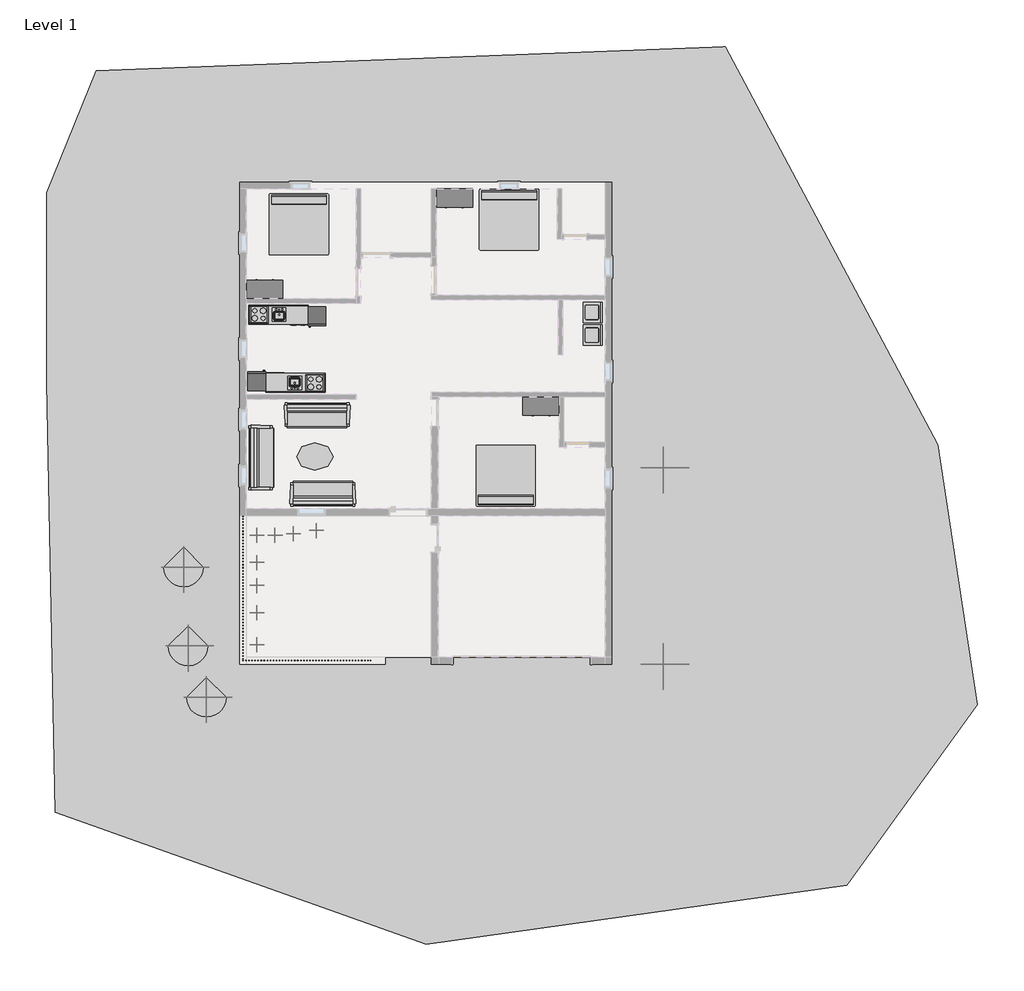
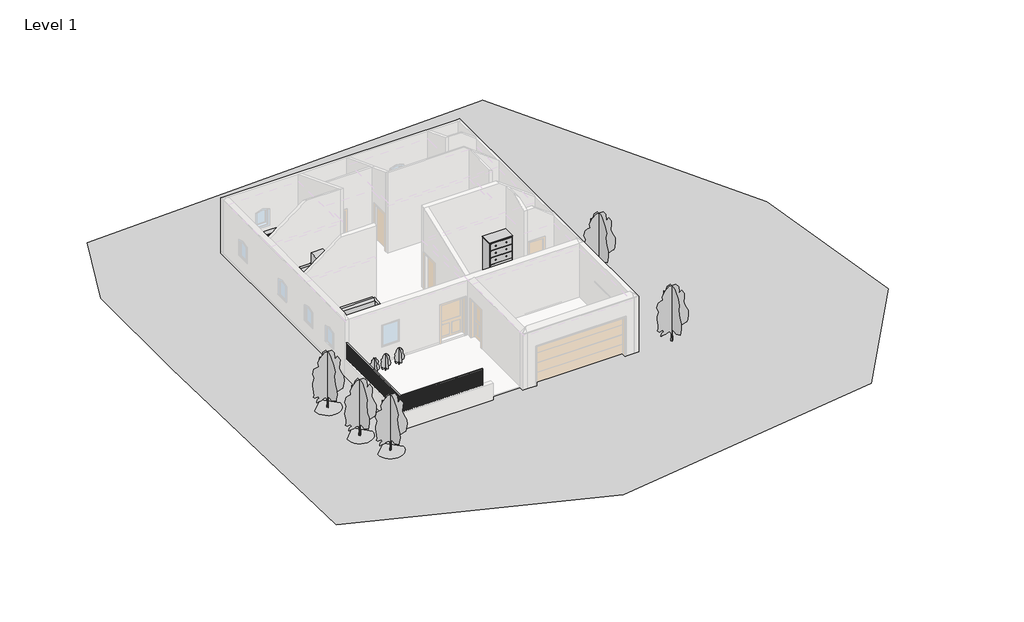
# One storey, part 3 of 3: 13 geographic elements, 12 furniture elements, 11 proxies, 2 flow terminals, 1 railing.
"""IFC4 building model written with IfcOpenShell, lengths in millimetres."""

from ifc_helpers import new_model, si_unit, frame, origin, place, context, project, spatial, polyline, outline, extrude, faceted_brep, triangles, transform, mapped, element, save
from components import proxy_a6faaae8, proxy_45b28599, kitchenette_medium_kitchenette_medium_844211aa, proxy_c523a7b7, proxy_718fa39f, flow_terminal_871c2e40, furniture_1fc5af50, furniture_c6510c7c, furniture_9fa109b2, furniture_aff9b2fb, furniture_b1c544a7, rpc_tree_deciduous_10_2_5dd3353f, rpc_tree_deciduous_red_ash_25_29d6c0be

model = new_model("IFC4")

# Units and contexts
model_context = context("Model", 3, world=origin())
ifc_project = project(units=[si_unit("LENGTHUNIT", "METRE", prefix="MILLI")], contexts=[model_context])

# Site, building, storey
site = spatial("IfcSite", under=ifc_project)
building = spatial("IfcBuilding", under=site)
storey = spatial("IfcBuildingStorey", under=building, Name="Level 1", Elevation=0.0)

# Proxies
placement = place(None, origin())
element("IfcBuildingElementProxy", 1, Name="Building Element Proxy", at=placement, inside=storey, context=model_context, shape_type="Tessellation", body=[
    triangles([(-17802.37034, 12771.1681366, 0.0), (3187.6458366, 13578.4769989, 0.0), (10269.9417389, 294.5849622, 0.0), (11590.9913361, -8365.631813, 0.0), (7224.187532, -14383.7487762, 0.0), (-6793.6207901, -16365.323172, 0.0), (-19160.1165344, -11961.8233521, 0.0), (-19453.6834991, 2386.2475147, 0.0), (-19453.6834991, 8697.9307159, 0.0)], [[2, 9, 8], [2, 1, 9], [8, 7, 6], [6, 5, 3], [3, 2, 8], [3, 5, 4], [3, 8, 6]], closed=False),
])
proxy_shape = proxy_a6faaae8(model_context)
element("IfcBuildingElementProxy", 2, Name="Cook Top-4 Unit2 : 22\" x 20\"", ObjectType="Cook Top-4 Unit2 : 22\" x 20\"", at=placement, inside=storey, context=model_context, shape_type="MappedRepresentation", body=[
    mapped(proxy_shape, transform((-12370.7368615, 4641.3670221, 152.4), x_axis=(1.0, 0.0, 0.0), y_axis=(0.0, 1.0, 0.0), z_axis=(0.0, 0.0, 1.0))),
])
element("IfcBuildingElementProxy", 3, Name="Cook Top-4 Unit2 : 22\" x 20\"", ObjectType="Cook Top-4 Unit2 : 22\" x 20\"", at=placement, inside=storey, context=model_context, shape_type="MappedRepresentation", body=[
    mapped(proxy_shape, transform((-10503.8368615, 2355.3670221, 152.4), x_axis=(-1.0, 0.0, 0.0), y_axis=(0.0, -1.0, 0.0), z_axis=(0.0, 0.0, 1.0))),
])
proxy_2_shape = proxy_45b28599(model_context)
element("IfcBuildingElementProxy", 4, Name="Dishwasher : 24\" x 24\" x 34\"", ObjectType="Dishwasher : 24\" x 24\" x 34\"", at=placement, inside=storey, context=model_context, shape_type="MappedRepresentation", body=[
    mapped(proxy_2_shape, transform((-11419.55433, 4349.5174573, 152.4), x_axis=(1.0, 0.0, 0.0), y_axis=(0.0, 1.0, 0.0), z_axis=(0.0, 0.0, 1.0))),
])
element("IfcBuildingElementProxy", 5, Name="Dishwasher : 24\" x 24\" x 34\"", ObjectType="Dishwasher : 24\" x 24\" x 34\"", at=placement, inside=storey, context=model_context, shape_type="MappedRepresentation", body=[
    mapped(proxy_2_shape, transform((-11455.019393, 2647.2165869, 152.4), x_axis=(-1.0, 0.0, 0.0), y_axis=(0.0, -1.0, 0.0), z_axis=(0.0, 0.0, 1.0))),
])
kitchenette_medium_kitchenette_medium_shape = kitchenette_medium_kitchenette_medium_844211aa(model_context)
element("IfcBuildingElementProxy", 6, Name="Kitchenette - Medium : Kitchenette - Medium", ObjectType="Kitchenette - Medium : Kitchenette - Medium", at=placement, inside=storey, context=model_context, shape_type="MappedRepresentation", body=[
    mapped(kitchenette_medium_kitchenette_medium_shape, transform((-12046.5745664, 4946.1670221, 152.4), x_axis=(1.0, 0.0, 0.0), y_axis=(0.0, 1.0, 0.0), z_axis=(0.0, 0.0, 1.0))),
])
element("IfcBuildingElementProxy", 7, Name="Kitchenette - Medium : Kitchenette - Medium", ObjectType="Kitchenette - Medium : Kitchenette - Medium", at=placement, inside=storey, context=model_context, shape_type="MappedRepresentation", body=[
    mapped(kitchenette_medium_kitchenette_medium_shape, transform((-10827.9991566, 2050.5670221, 152.4), x_axis=(-1.0, 0.0, 0.0), y_axis=(0.0, -1.0, 0.0), z_axis=(0.0, 0.0, 1.0))),
])
proxy_3_shape = proxy_c523a7b7(model_context)
element("IfcBuildingElementProxy", 8, Name="Refrigerator : 24\" x 25\" LH", ObjectType="Refrigerator : 24\" x 25\" LH", at=placement, inside=storey, context=model_context, shape_type="MappedRepresentation", body=[
    mapped(proxy_3_shape, transform((-10433.9868615, 4595.7180506, 152.4), x_axis=(1.0, 0.0, 0.0), y_axis=(0.0, 1.0, 0.0), z_axis=(0.0, 0.0, 1.0))),
])
element("IfcBuildingElementProxy", 9, Name="Refrigerator : 24\" x 25\" LH", ObjectType="Refrigerator : 24\" x 25\" LH", at=placement, inside=storey, context=model_context, shape_type="MappedRepresentation", body=[
    mapped(proxy_3_shape, transform((-12440.5868615, 2401.0159936, 152.4), x_axis=(-1.0, 0.0, 0.0), y_axis=(0.0, -1.0, 0.0), z_axis=(0.0, 0.0, 1.0))),
])
proxy_4_shape = proxy_718fa39f(model_context)
element("IfcBuildingElementProxy", 10, Name="Washer : 27\" x 25\" x 35\"", ObjectType="Washer : 27\" x 25\" x 35\"", at=placement, inside=storey, context=model_context, shape_type="MappedRepresentation", body=[
    mapped(proxy_4_shape, transform((-1511.9864263, 5136.6670221, 152.4), x_axis=(0.0, -1.0, 0.0), y_axis=(1.0, 0.0, 0.0), z_axis=(0.0, 0.0, 1.0))),
])
element("IfcBuildingElementProxy", 11, Name="Washer : 27\" x 25\" x 35\"", ObjectType="Washer : 27\" x 25\" x 35\"", at=placement, inside=storey, context=model_context, shape_type="MappedRepresentation", body=[
    mapped(proxy_4_shape, transform((-1511.9864263, 4373.3495536, 152.4), x_axis=(0.0, -1.0, 0.0), y_axis=(1.0, 0.0, 0.0), z_axis=(0.0, 0.0, 1.0))),
])

# Flow terminals
flow_terminal_shape = flow_terminal_871c2e40(model_context)
element("IfcFlowTerminal", 12, ObjectType="Sink Kitchen-Island : 18\" x 18\"", at=placement, inside=storey, context=model_context, shape_type="MappedRepresentation", body=[
    mapped(flow_terminal_shape, transform((-11713.3261021, 4639.021621, 138.0), x_axis=(1.0, 0.0, 0.0), y_axis=(0.0, 1.0, 0.0), z_axis=(0.0, 0.0, 1.0))),
])
element("IfcFlowTerminal", 13, ObjectType="Sink Kitchen-Island : 18\" x 18\"", at=placement, inside=storey, context=model_context, shape_type="MappedRepresentation", body=[
    mapped(flow_terminal_shape, transform((-11161.2476209, 2357.7124232, 138.0), x_axis=(-1.0, 0.0, 0.0), y_axis=(0.0, -1.0, 0.0), z_axis=(0.0, 0.0, 1.0))),
])

# Furniture
furniture_shape = furniture_1fc5af50(model_context)
element("IfcFurniture", 14, ObjectType="Bed-Standard : King 78\" x 80\"", at=placement, inside=storey, context=model_context, shape_type="MappedRepresentation", body=[
    mapped(furniture_shape, transform((-11308.7253861, 7696.8621041, 152.4), x_axis=(1.0, 0.0, 0.0), y_axis=(0.0, 1.0, 0.0), z_axis=(0.0, 0.0, 1.0))),
])
element("IfcFurniture", 15, ObjectType="Bed-Standard : King 78\" x 80\"", at=placement, inside=storey, context=model_context, shape_type="MappedRepresentation", body=[
    mapped(furniture_shape, transform((-4298.3253861, 7849.2621041, 152.4), x_axis=(1.0, 0.0, 0.0), y_axis=(0.0, 1.0, 0.0), z_axis=(0.0, 0.0, 1.0))),
])
element("IfcFurniture", 16, ObjectType="Bed-Standard : King 78\" x 80\"", at=placement, inside=storey, context=model_context, shape_type="MappedRepresentation", body=[
    mapped(furniture_shape, transform((-3869.6483369, -776.3280599, 152.4), x_axis=(-1.0000000000000002, 0.0, 0.0), y_axis=(0.0, -1.0000000000000002, 0.0), z_axis=(0.0, 0.0, 1.0))),
])
furniture_2_shape = furniture_c6510c7c(model_context)
element("IfcFurniture", 17, ObjectType="Counter Top w Sink Hole : 24\" Depth", at=placement, inside=storey, context=model_context, shape_type="MappedRepresentation", body=[
    mapped(furniture_2_shape, transform((-11513.1745664, 4946.1670221, 138.0), x_axis=(1.0, 0.0, 0.0), y_axis=(0.0, 1.0, 0.0), z_axis=(0.0, 0.0, 1.0))),
])
element("IfcFurniture", 18, ObjectType="Counter Top w Sink Hole : 24\" Depth", at=placement, inside=storey, context=model_context, shape_type="MappedRepresentation", body=[
    mapped(furniture_2_shape, transform((-11361.3991566, 2050.5670221, 138.0), x_axis=(-1.0, 0.0, 0.0), y_axis=(0.0, -1.0, 0.0), z_axis=(0.0, 0.0, 1.0))),
])
furniture_3_shape = furniture_9fa109b2(model_context)
element("IfcFurniture", 19, ObjectType="Dresser : 48\" x 72\" x 24\"", at=placement, inside=storey, context=model_context, shape_type="MappedRepresentation", body=[
    mapped(furniture_3_shape, transform((-12449.4301213, 5116.404068, 152.4), x_axis=(-1.0000000000000004, 0.0, 0.0), y_axis=(0.0, -1.0000000000000004, 0.0), z_axis=(0.0, 0.0, 1.0))),
])
element("IfcFurniture", 20, ObjectType="Dresser : 48\" x 72\" x 24\"", at=placement, inside=storey, context=model_context, shape_type="MappedRepresentation", body=[
    mapped(furniture_3_shape, transform((-5586.4436017, 8890.7299762, 152.4), x_axis=(1.0000000000000004, 0.0, 0.0), y_axis=(0.0, 1.0000000000000004, 0.0), z_axis=(0.0, 0.0, 1.0))),
])
element("IfcFurniture", 21, ObjectType="Dresser : 48\" x 72\" x 24\"", at=placement, inside=storey, context=model_context, shape_type="MappedRepresentation", body=[
    mapped(furniture_3_shape, transform((-2690.8436017, 1956.5299762, 152.4), x_axis=(1.0000000000000004, 0.0, 0.0), y_axis=(0.0, 1.0000000000000004, 0.0), z_axis=(0.0, 0.0, 1.0))),
])
furniture_4_shape = furniture_aff9b2fb(model_context)
element("IfcFurniture", 22, ObjectType="Sofa-Pensi : 84\"", at=placement, inside=storey, context=model_context, shape_type="MappedRepresentation", body=[
    mapped(furniture_4_shape, transform((-12017.4270254, -412.4392279, 152.4), x_axis=(0.0, 1.0000000000000002, 0.0), y_axis=(-1.0000000000000002, 0.0, 0.0), z_axis=(0.0, 0.0, 1.0))),
])
element("IfcFurniture", 23, ObjectType="Sofa-Pensi : 84\"", at=placement, inside=storey, context=model_context, shape_type="MappedRepresentation", body=[
    mapped(furniture_4_shape, transform((-10706.2431115, 1011.457186, 152.4), x_axis=(1.0000000000000007, 0.0, 0.0), y_axis=(0.0, 1.0000000000000007, 0.0), z_axis=(0.0, 0.0, 1.0))),
])
element("IfcFurniture", 24, ObjectType="Sofa-Pensi : 84\"", at=placement, inside=storey, context=model_context, shape_type="MappedRepresentation", body=[
    mapped(furniture_4_shape, transform((-9958.5306115, -1063.2231418, 152.4), x_axis=(-1.0000000000000004, 0.0, 0.0), y_axis=(0.0, -1.0000000000000004, 0.0), z_axis=(0.0, 0.0, 1.0))),
])
furniture_5_shape = furniture_b1c544a7(model_context)
element("IfcFurniture", 25, ObjectType="Table-Ellipse : 60\" x 48\"", at=placement, inside=storey, context=model_context, shape_type="MappedRepresentation", body=[
    mapped(furniture_5_shape, transform((-10503.8368615, -95.7329779, 152.4), x_axis=(0.0, -1.0000000000000004, 0.0), y_axis=(1.0000000000000004, 0.0, 0.0), z_axis=(0.0, 0.0, 1.0))),
])

# Geographic elements
rpc_tree_deciduous_10_2_shape = rpc_tree_deciduous_10_2_5dd3353f(model_context)
element("IfcGeographicElement", 26, ObjectType="RPC Tree - Deciduous : 10' 2", at=placement, inside=storey, context=model_context, shape_type="MappedRepresentation", body=[
    mapped(rpc_tree_deciduous_10_2_shape, transform((-14885.3368615, -3778.7329779, 0.0), x_axis=(1.0, 0.0, 0.0), y_axis=(0.0, 1.0, 0.0), z_axis=(0.0, 0.0, 1.0))),
])
element("IfcGeographicElement", 27, ObjectType="RPC Tree - Deciduous : 10' 2", at=placement, inside=storey, context=model_context, shape_type="MappedRepresentation", body=[
    mapped(rpc_tree_deciduous_10_2_shape, transform((-14732.9368615, -6407.6329779, 0.0), x_axis=(1.0, 0.0, 0.0), y_axis=(0.0, 1.0, 0.0), z_axis=(0.0, 0.0, 1.0))),
])
element("IfcGeographicElement", 28, ObjectType="RPC Tree - Deciduous : 10' 2", at=placement, inside=storey, context=model_context, shape_type="MappedRepresentation", body=[
    mapped(rpc_tree_deciduous_10_2_shape, transform((1116.6631385, -7017.2329779, 0.0), x_axis=(1.0, 0.0, 0.0), y_axis=(0.0, 1.0, 0.0), z_axis=(0.0, 0.0, 1.0))),
])
element("IfcGeographicElement", 29, ObjectType="RPC Tree - Deciduous : 10' 2", at=placement, inside=storey, context=model_context, shape_type="MappedRepresentation", body=[
    mapped(rpc_tree_deciduous_10_2_shape, transform((1116.6631385, -464.0329779, 0.0), x_axis=(1.0, 0.0, 0.0), y_axis=(0.0, 1.0, 0.0), z_axis=(0.0, 0.0, 1.0))),
])
element("IfcGeographicElement", 30, ObjectType="RPC Tree - Deciduous : 10' 2", at=placement, inside=storey, context=model_context, shape_type="MappedRepresentation", body=[
    mapped(rpc_tree_deciduous_10_2_shape, transform((-14123.3368615, -8122.1329779, 0.0), x_axis=(1.0, 0.0, 0.0), y_axis=(0.0, 1.0, 0.0), z_axis=(0.0, 0.0, 1.0))),
])
rpc_tree_deciduous_red_ash_25_shape = rpc_tree_deciduous_red_ash_25_29d6c0be(model_context)
element("IfcGeographicElement", 31, ObjectType="RPC Tree - Deciduous : Red Ash - 25'", at=placement, inside=storey, context=model_context, shape_type="MappedRepresentation", body=[
    mapped(rpc_tree_deciduous_red_ash_25_shape, transform((-12446.9368615, -2711.9329779, 50.8), x_axis=(1.0, 0.0, 0.0), y_axis=(0.0, 1.0, 0.0), z_axis=(0.0, 0.0, 1.0))),
])
element("IfcGeographicElement", 32, ObjectType="RPC Tree - Deciduous : Red Ash - 25'", at=placement, inside=storey, context=model_context, shape_type="MappedRepresentation", body=[
    mapped(rpc_tree_deciduous_red_ash_25_shape, transform((-12446.9368615, -3626.3329779, 50.8), x_axis=(1.0, 0.0, 0.0), y_axis=(0.0, 1.0, 0.0), z_axis=(0.0, 0.0, 1.0))),
])
element("IfcGeographicElement", 33, ObjectType="RPC Tree - Deciduous : Red Ash - 25'", at=placement, inside=storey, context=model_context, shape_type="MappedRepresentation", body=[
    mapped(rpc_tree_deciduous_red_ash_25_shape, transform((-12446.9368615, -4388.3329779, 50.8), x_axis=(1.0, 0.0, 0.0), y_axis=(0.0, 1.0, 0.0), z_axis=(0.0, 0.0, 1.0))),
])
element("IfcGeographicElement", 34, ObjectType="RPC Tree - Deciduous : Red Ash - 25'", at=placement, inside=storey, context=model_context, shape_type="MappedRepresentation", body=[
    mapped(rpc_tree_deciduous_red_ash_25_shape, transform((-12446.9368615, -5302.7329779, 50.8), x_axis=(1.0, 0.0, 0.0), y_axis=(0.0, 1.0, 0.0), z_axis=(0.0, 0.0, 1.0))),
])
element("IfcGeographicElement", 35, ObjectType="RPC Tree - Deciduous : Red Ash - 25'", at=placement, inside=storey, context=model_context, shape_type="MappedRepresentation", body=[
    mapped(rpc_tree_deciduous_red_ash_25_shape, transform((-12446.9368615, -6369.5329779, 50.8), x_axis=(1.0, 0.0, 0.0), y_axis=(0.0, 1.0, 0.0), z_axis=(0.0, 0.0, 1.0))),
])
element("IfcGeographicElement", 36, ObjectType="RPC Tree - Deciduous : Red Ash - 25'", at=placement, inside=storey, context=model_context, shape_type="MappedRepresentation", body=[
    mapped(rpc_tree_deciduous_red_ash_25_shape, transform((-11837.3368615, -2711.9329779, 50.8), x_axis=(1.0, 0.0, 0.0), y_axis=(0.0, 1.0, 0.0), z_axis=(0.0, 0.0, 1.0))),
])
element("IfcGeographicElement", 37, ObjectType="RPC Tree - Deciduous : Red Ash - 25'", at=placement, inside=storey, context=model_context, shape_type="MappedRepresentation", body=[
    mapped(rpc_tree_deciduous_red_ash_25_shape, transform((-11227.7368615, -2661.1329779, 50.8), x_axis=(1.0, 0.0, 0.0), y_axis=(0.0, 1.0, 0.0), z_axis=(0.0, 0.0, 1.0))),
])
element("IfcGeographicElement", 38, ObjectType="RPC Tree - Deciduous : Red Ash - 25'", at=placement, inside=storey, context=model_context, shape_type="MappedRepresentation", body=[
    mapped(rpc_tree_deciduous_red_ash_25_shape, transform((-10465.7368615, -2559.5329779, 50.8), x_axis=(1.0, 0.0, 0.0), y_axis=(0.0, 1.0, 0.0), z_axis=(0.0, 0.0, 1.0))),
])

# Railing
element("IfcRailing", 39, ObjectType="Handrail - Rectangular", at=placement, inside=storey, context=model_context, shape_type="SolidModel", body=[
    faceted_brep([(-12878.7368615, -2076.9329779, 1828.8), (-12878.7368615, -2076.9329779, 1778.0), (-12929.5368615, -2076.9329779, 1778.0), (-12929.5368615, -2076.9329779, 1828.8), (-12878.7368615, -6877.5329779, 1828.8), (-12878.7368615, -6877.5329779, 1778.0), (-12929.5368615, -6928.3329779, 1778.0), (-12929.5368615, -6928.3329779, 1828.8), (-8636.9368615, -6877.5329779, 1828.8), (-8636.9368615, -6928.3329779, 1828.8), (-8636.9368615, -6928.3329779, 1778.0), (-8636.9368615, -6877.5329779, 1778.0)], [[[0, 1, 2, 3]], [[1, 0, 4, 5]], [[2, 1, 5, 6]], [[3, 2, 6, 7]], [[0, 3, 7, 4]], [[8, 9, 10, 11]], [[5, 4, 8, 11]], [[6, 5, 11, 10]], [[7, 6, 10, 9]], [[4, 7, 9, 8]]]),
    extrude(outline(polyline([(-8748.0618615, -6912.4579779), (-8748.0618615, -6893.4079779), (-8729.0118615, -6893.4079779), (-8729.0118615, -6912.4579779), (-8748.0618615, -6912.4579779)])), frame((0.0, 0.0, 914.4), z_axis=(0.0, 0.0, 1.0), x_axis=(1.0, 0.0, 0.0)), (0.0, 0.0, 1.0), 863.6),
    extrude(outline(polyline([(-8849.6618615, -6912.4579779), (-8849.6618615, -6893.4079779), (-8830.6118615, -6893.4079779), (-8830.6118615, -6912.4579779), (-8849.6618615, -6912.4579779)])), frame((0.0, 0.0, 914.4), z_axis=(0.0, 0.0, 1.0), x_axis=(1.0, 0.0, 0.0)), (0.0, 0.0, 1.0), 863.6),
    extrude(outline(polyline([(-8951.2618615, -6912.4579779), (-8951.2618615, -6893.4079779), (-8932.2118615, -6893.4079779), (-8932.2118615, -6912.4579779), (-8951.2618615, -6912.4579779)])), frame((0.0, 0.0, 914.4), z_axis=(0.0, 0.0, 1.0), x_axis=(1.0, 0.0, 0.0)), (0.0, 0.0, 1.0), 863.6),
    extrude(outline(polyline([(-9052.8618615, -6912.4579779), (-9052.8618615, -6893.4079779), (-9033.8118615, -6893.4079779), (-9033.8118615, -6912.4579779), (-9052.8618615, -6912.4579779)])), frame((0.0, 0.0, 914.4), z_axis=(0.0, 0.0, 1.0), x_axis=(1.0, 0.0, 0.0)), (0.0, 0.0, 1.0), 863.6),
    extrude(outline(polyline([(-9154.4618615, -6912.4579779), (-9154.4618615, -6893.4079779), (-9135.4118615, -6893.4079779), (-9135.4118615, -6912.4579779), (-9154.4618615, -6912.4579779)])), frame((0.0, 0.0, 914.4), z_axis=(0.0, 0.0, 1.0), x_axis=(1.0, 0.0, 0.0)), (0.0, 0.0, 1.0), 863.6),
    extrude(outline(polyline([(-9256.0618615, -6912.4579779), (-9256.0618615, -6893.4079779), (-9237.0118615, -6893.4079779), (-9237.0118615, -6912.4579779), (-9256.0618615, -6912.4579779)])), frame((0.0, 0.0, 914.4), z_axis=(0.0, 0.0, 1.0), x_axis=(1.0, 0.0, 0.0)), (0.0, 0.0, 1.0), 863.6),
    extrude(outline(polyline([(-9357.6618615, -6912.4579779), (-9357.6618615, -6893.4079779), (-9338.6118615, -6893.4079779), (-9338.6118615, -6912.4579779), (-9357.6618615, -6912.4579779)])), frame((0.0, 0.0, 914.4), z_axis=(0.0, 0.0, 1.0), x_axis=(1.0, 0.0, 0.0)), (0.0, 0.0, 1.0), 863.6),
    extrude(outline(polyline([(-9459.2618615, -6912.4579779), (-9459.2618615, -6893.4079779), (-9440.2118615, -6893.4079779), (-9440.2118615, -6912.4579779), (-9459.2618615, -6912.4579779)])), frame((0.0, 0.0, 914.4), z_axis=(0.0, 0.0, 1.0), x_axis=(1.0, 0.0, 0.0)), (0.0, 0.0, 1.0), 863.6),
    extrude(outline(polyline([(-9560.8618615, -6912.4579779), (-9560.8618615, -6893.4079779), (-9541.8118615, -6893.4079779), (-9541.8118615, -6912.4579779), (-9560.8618615, -6912.4579779)])), frame((0.0, 0.0, 914.4), z_axis=(0.0, 0.0, 1.0), x_axis=(1.0, 0.0, 0.0)), (0.0, 0.0, 1.0), 863.6),
    extrude(outline(polyline([(-9662.4618615, -6912.4579779), (-9662.4618615, -6893.4079779), (-9643.4118615, -6893.4079779), (-9643.4118615, -6912.4579779), (-9662.4618615, -6912.4579779)])), frame((0.0, 0.0, 914.4), z_axis=(0.0, 0.0, 1.0), x_axis=(1.0, 0.0, 0.0)), (0.0, 0.0, 1.0), 863.6),
    extrude(outline(polyline([(-9764.0618615, -6912.4579779), (-9764.0618615, -6893.4079779), (-9745.0118615, -6893.4079779), (-9745.0118615, -6912.4579779), (-9764.0618615, -6912.4579779)])), frame((0.0, 0.0, 914.4), z_axis=(0.0, 0.0, 1.0), x_axis=(1.0, 0.0, 0.0)), (0.0, 0.0, 1.0), 863.6),
    extrude(outline(polyline([(-9865.6618615, -6912.4579779), (-9865.6618615, -6893.4079779), (-9846.6118615, -6893.4079779), (-9846.6118615, -6912.4579779), (-9865.6618615, -6912.4579779)])), frame((0.0, 0.0, 914.4), z_axis=(0.0, 0.0, 1.0), x_axis=(1.0, 0.0, 0.0)), (0.0, 0.0, 1.0), 863.6),
    extrude(outline(polyline([(-9967.2618615, -6912.4579779), (-9967.2618615, -6893.4079779), (-9948.2118615, -6893.4079779), (-9948.2118615, -6912.4579779), (-9967.2618615, -6912.4579779)])), frame((0.0, 0.0, 914.4), z_axis=(0.0, 0.0, 1.0), x_axis=(1.0, 0.0, 0.0)), (0.0, 0.0, 1.0), 863.6),
    extrude(outline(polyline([(-10068.8618615, -6912.4579779), (-10068.8618615, -6893.4079779), (-10049.8118615, -6893.4079779), (-10049.8118615, -6912.4579779), (-10068.8618615, -6912.4579779)])), frame((0.0, 0.0, 914.4), z_axis=(0.0, 0.0, 1.0), x_axis=(1.0, 0.0, 0.0)), (0.0, 0.0, 1.0), 863.6),
    extrude(outline(polyline([(-10170.4618615, -6912.4579779), (-10170.4618615, -6893.4079779), (-10151.4118615, -6893.4079779), (-10151.4118615, -6912.4579779), (-10170.4618615, -6912.4579779)])), frame((0.0, 0.0, 914.4), z_axis=(0.0, 0.0, 1.0), x_axis=(1.0, 0.0, 0.0)), (0.0, 0.0, 1.0), 863.6),
    extrude(outline(polyline([(-10272.0618615, -6912.4579779), (-10272.0618615, -6893.4079779), (-10253.0118615, -6893.4079779), (-10253.0118615, -6912.4579779), (-10272.0618615, -6912.4579779)])), frame((0.0, 0.0, 914.4), z_axis=(0.0, 0.0, 1.0), x_axis=(1.0, 0.0, 0.0)), (0.0, 0.0, 1.0), 863.6),
    extrude(outline(polyline([(-10373.6618615, -6912.4579779), (-10373.6618615, -6893.4079779), (-10354.6118615, -6893.4079779), (-10354.6118615, -6912.4579779), (-10373.6618615, -6912.4579779)])), frame((0.0, 0.0, 914.4), z_axis=(0.0, 0.0, 1.0), x_axis=(1.0, 0.0, 0.0)), (0.0, 0.0, 1.0), 863.6),
    extrude(outline(polyline([(-10475.2618615, -6912.4579779), (-10475.2618615, -6893.4079779), (-10456.2118615, -6893.4079779), (-10456.2118615, -6912.4579779), (-10475.2618615, -6912.4579779)])), frame((0.0, 0.0, 914.4), z_axis=(0.0, 0.0, 1.0), x_axis=(1.0, 0.0, 0.0)), (0.0, 0.0, 1.0), 863.6),
    extrude(outline(polyline([(-10576.8618615, -6912.4579779), (-10576.8618615, -6893.4079779), (-10557.8118615, -6893.4079779), (-10557.8118615, -6912.4579779), (-10576.8618615, -6912.4579779)])), frame((0.0, 0.0, 914.4), z_axis=(0.0, 0.0, 1.0), x_axis=(1.0, 0.0, 0.0)), (0.0, 0.0, 1.0), 863.6),
    extrude(outline(polyline([(-10678.4618615, -6912.4579779), (-10678.4618615, -6893.4079779), (-10659.4118615, -6893.4079779), (-10659.4118615, -6912.4579779), (-10678.4618615, -6912.4579779)])), frame((0.0, 0.0, 914.4), z_axis=(0.0, 0.0, 1.0), x_axis=(1.0, 0.0, 0.0)), (0.0, 0.0, 1.0), 863.6),
    extrude(outline(polyline([(-10780.0618615, -6912.4579779), (-10780.0618615, -6893.4079779), (-10761.0118615, -6893.4079779), (-10761.0118615, -6912.4579779), (-10780.0618615, -6912.4579779)])), frame((0.0, 0.0, 914.4), z_axis=(0.0, 0.0, 1.0), x_axis=(1.0, 0.0, 0.0)), (0.0, 0.0, 1.0), 863.6),
    extrude(outline(polyline([(-10881.6618615, -6912.4579779), (-10881.6618615, -6893.4079779), (-10862.6118615, -6893.4079779), (-10862.6118615, -6912.4579779), (-10881.6618615, -6912.4579779)])), frame((0.0, 0.0, 914.4), z_axis=(0.0, 0.0, 1.0), x_axis=(1.0, 0.0, 0.0)), (0.0, 0.0, 1.0), 863.6),
    extrude(outline(polyline([(-10983.2618615, -6912.4579779), (-10983.2618615, -6893.4079779), (-10964.2118615, -6893.4079779), (-10964.2118615, -6912.4579779), (-10983.2618615, -6912.4579779)])), frame((0.0, 0.0, 914.4), z_axis=(0.0, 0.0, 1.0), x_axis=(1.0, 0.0, 0.0)), (0.0, 0.0, 1.0), 863.6),
    extrude(outline(polyline([(-11084.8618615, -6912.4579779), (-11084.8618615, -6893.4079779), (-11065.8118615, -6893.4079779), (-11065.8118615, -6912.4579779), (-11084.8618615, -6912.4579779)])), frame((0.0, 0.0, 914.4), z_axis=(0.0, 0.0, 1.0), x_axis=(1.0, 0.0, 0.0)), (0.0, 0.0, 1.0), 863.6),
    extrude(outline(polyline([(-11186.4618615, -6912.4579779), (-11186.4618615, -6893.4079779), (-11167.4118615, -6893.4079779), (-11167.4118615, -6912.4579779), (-11186.4618615, -6912.4579779)])), frame((0.0, 0.0, 914.4), z_axis=(0.0, 0.0, 1.0), x_axis=(1.0, 0.0, 0.0)), (0.0, 0.0, 1.0), 863.6),
    extrude(outline(polyline([(-11288.0618615, -6912.4579779), (-11288.0618615, -6893.4079779), (-11269.0118615, -6893.4079779), (-11269.0118615, -6912.4579779), (-11288.0618615, -6912.4579779)])), frame((0.0, 0.0, 914.4), z_axis=(0.0, 0.0, 1.0), x_axis=(1.0, 0.0, 0.0)), (0.0, 0.0, 1.0), 863.6),
    extrude(outline(polyline([(-11389.6618615, -6912.4579779), (-11389.6618615, -6893.4079779), (-11370.6118615, -6893.4079779), (-11370.6118615, -6912.4579779), (-11389.6618615, -6912.4579779)])), frame((0.0, 0.0, 914.4), z_axis=(0.0, 0.0, 1.0), x_axis=(1.0, 0.0, 0.0)), (0.0, 0.0, 1.0), 863.6),
    extrude(outline(polyline([(-11491.2618615, -6912.4579779), (-11491.2618615, -6893.4079779), (-11472.2118615, -6893.4079779), (-11472.2118615, -6912.4579779), (-11491.2618615, -6912.4579779)])), frame((0.0, 0.0, 914.4), z_axis=(0.0, 0.0, 1.0), x_axis=(1.0, 0.0, 0.0)), (0.0, 0.0, 1.0), 863.6),
    extrude(outline(polyline([(-11592.8618615, -6912.4579779), (-11592.8618615, -6893.4079779), (-11573.8118615, -6893.4079779), (-11573.8118615, -6912.4579779), (-11592.8618615, -6912.4579779)])), frame((0.0, 0.0, 914.4), z_axis=(0.0, 0.0, 1.0), x_axis=(1.0, 0.0, 0.0)), (0.0, 0.0, 1.0), 863.6),
    extrude(outline(polyline([(-11694.4618615, -6912.4579779), (-11694.4618615, -6893.4079779), (-11675.4118615, -6893.4079779), (-11675.4118615, -6912.4579779), (-11694.4618615, -6912.4579779)])), frame((0.0, 0.0, 914.4), z_axis=(0.0, 0.0, 1.0), x_axis=(1.0, 0.0, 0.0)), (0.0, 0.0, 1.0), 863.6),
    extrude(outline(polyline([(-11796.0618615, -6912.4579779), (-11796.0618615, -6893.4079779), (-11777.0118615, -6893.4079779), (-11777.0118615, -6912.4579779), (-11796.0618615, -6912.4579779)])), frame((0.0, 0.0, 914.4), z_axis=(0.0, 0.0, 1.0), x_axis=(1.0, 0.0, 0.0)), (0.0, 0.0, 1.0), 863.6),
    extrude(outline(polyline([(-11897.6618615, -6912.4579779), (-11897.6618615, -6893.4079779), (-11878.6118615, -6893.4079779), (-11878.6118615, -6912.4579779), (-11897.6618615, -6912.4579779)])), frame((0.0, 0.0, 914.4), z_axis=(0.0, 0.0, 1.0), x_axis=(1.0, 0.0, 0.0)), (0.0, 0.0, 1.0), 863.6),
    extrude(outline(polyline([(-11999.2618615, -6912.4579779), (-11999.2618615, -6893.4079779), (-11980.2118615, -6893.4079779), (-11980.2118615, -6912.4579779), (-11999.2618615, -6912.4579779)])), frame((0.0, 0.0, 914.4), z_axis=(0.0, 0.0, 1.0), x_axis=(1.0, 0.0, 0.0)), (0.0, 0.0, 1.0), 863.6),
    extrude(outline(polyline([(-12100.8618615, -6912.4579779), (-12100.8618615, -6893.4079779), (-12081.8118615, -6893.4079779), (-12081.8118615, -6912.4579779), (-12100.8618615, -6912.4579779)])), frame((0.0, 0.0, 914.4), z_axis=(0.0, 0.0, 1.0), x_axis=(1.0, 0.0, 0.0)), (0.0, 0.0, 1.0), 863.6),
    extrude(outline(polyline([(-12202.4618615, -6912.4579779), (-12202.4618615, -6893.4079779), (-12183.4118615, -6893.4079779), (-12183.4118615, -6912.4579779), (-12202.4618615, -6912.4579779)])), frame((0.0, 0.0, 914.4), z_axis=(0.0, 0.0, 1.0), x_axis=(1.0, 0.0, 0.0)), (0.0, 0.0, 1.0), 863.6),
    extrude(outline(polyline([(-12304.0618615, -6912.4579779), (-12304.0618615, -6893.4079779), (-12285.0118615, -6893.4079779), (-12285.0118615, -6912.4579779), (-12304.0618615, -6912.4579779)])), frame((0.0, 0.0, 914.4), z_axis=(0.0, 0.0, 1.0), x_axis=(1.0, 0.0, 0.0)), (0.0, 0.0, 1.0), 863.6),
    extrude(outline(polyline([(-12405.6618615, -6912.4579779), (-12405.6618615, -6893.4079779), (-12386.6118615, -6893.4079779), (-12386.6118615, -6912.4579779), (-12405.6618615, -6912.4579779)])), frame((0.0, 0.0, 914.4), z_axis=(0.0, 0.0, 1.0), x_axis=(1.0, 0.0, 0.0)), (0.0, 0.0, 1.0), 863.6),
    extrude(outline(polyline([(-12507.2618615, -6912.4579779), (-12507.2618615, -6893.4079779), (-12488.2118615, -6893.4079779), (-12488.2118615, -6912.4579779), (-12507.2618615, -6912.4579779)])), frame((0.0, 0.0, 914.4), z_axis=(0.0, 0.0, 1.0), x_axis=(1.0, 0.0, 0.0)), (0.0, 0.0, 1.0), 863.6),
    extrude(outline(polyline([(-12608.8618615, -6912.4579779), (-12608.8618615, -6893.4079779), (-12589.8118615, -6893.4079779), (-12589.8118615, -6912.4579779), (-12608.8618615, -6912.4579779)])), frame((0.0, 0.0, 914.4), z_axis=(0.0, 0.0, 1.0), x_axis=(1.0, 0.0, 0.0)), (0.0, 0.0, 1.0), 863.6),
    extrude(outline(polyline([(-12710.4618615, -6912.4579779), (-12710.4618615, -6893.4079779), (-12691.4118615, -6893.4079779), (-12691.4118615, -6912.4579779), (-12710.4618615, -6912.4579779)])), frame((0.0, 0.0, 914.4), z_axis=(0.0, 0.0, 1.0), x_axis=(1.0, 0.0, 0.0)), (0.0, 0.0, 1.0), 863.6),
    extrude(outline(polyline([(-12812.0618615, -6912.4579779), (-12812.0618615, -6893.4079779), (-12793.0118615, -6893.4079779), (-12793.0118615, -6912.4579779), (-12812.0618615, -6912.4579779)])), frame((0.0, 0.0, 914.4), z_axis=(0.0, 0.0, 1.0), x_axis=(1.0, 0.0, 0.0)), (0.0, 0.0, 1.0), 863.6),
    extrude(outline(polyline([(-12913.6618615, -6842.6079779), (-12894.6118615, -6842.6079779), (-12894.6118615, -6861.6579779), (-12913.6618615, -6861.6579779), (-12913.6618615, -6842.6079779)])), frame((0.0, 0.0, 914.4), z_axis=(0.0, 0.0, 1.0), x_axis=(1.0, 0.0, 0.0)), (0.0, 0.0, 1.0), 863.6),
    extrude(outline(polyline([(-12913.6618615, -6741.0079779), (-12894.6118615, -6741.0079779), (-12894.6118615, -6760.0579779), (-12913.6618615, -6760.0579779), (-12913.6618615, -6741.0079779)])), frame((0.0, 0.0, 914.4), z_axis=(0.0, 0.0, 1.0), x_axis=(1.0, 0.0, 0.0)), (0.0, 0.0, 1.0), 863.6),
    extrude(outline(polyline([(-12913.6618615, -6639.4079779), (-12894.6118615, -6639.4079779), (-12894.6118615, -6658.4579779), (-12913.6618615, -6658.4579779), (-12913.6618615, -6639.4079779)])), frame((0.0, 0.0, 914.4), z_axis=(0.0, 0.0, 1.0), x_axis=(1.0, 0.0, 0.0)), (0.0, 0.0, 1.0), 863.6),
    extrude(outline(polyline([(-12913.6618615, -6537.8079779), (-12894.6118615, -6537.8079779), (-12894.6118615, -6556.8579779), (-12913.6618615, -6556.8579779), (-12913.6618615, -6537.8079779)])), frame((0.0, 0.0, 914.4), z_axis=(0.0, 0.0, 1.0), x_axis=(1.0, 0.0, 0.0)), (0.0, 0.0, 1.0), 863.6),
    extrude(outline(polyline([(-12913.6618615, -6436.2079779), (-12894.6118615, -6436.2079779), (-12894.6118615, -6455.2579779), (-12913.6618615, -6455.2579779), (-12913.6618615, -6436.2079779)])), frame((0.0, 0.0, 914.4), z_axis=(0.0, 0.0, 1.0), x_axis=(1.0, 0.0, 0.0)), (0.0, 0.0, 1.0), 863.6),
    extrude(outline(polyline([(-12913.6618615, -6334.6079779), (-12894.6118615, -6334.6079779), (-12894.6118615, -6353.6579779), (-12913.6618615, -6353.6579779), (-12913.6618615, -6334.6079779)])), frame((0.0, 0.0, 914.4), z_axis=(0.0, 0.0, 1.0), x_axis=(1.0, 0.0, 0.0)), (0.0, 0.0, 1.0), 863.6),
    extrude(outline(polyline([(-12913.6618615, -6233.0079779), (-12894.6118615, -6233.0079779), (-12894.6118615, -6252.0579779), (-12913.6618615, -6252.0579779), (-12913.6618615, -6233.0079779)])), frame((0.0, 0.0, 914.4), z_axis=(0.0, 0.0, 1.0), x_axis=(1.0, 0.0, 0.0)), (0.0, 0.0, 1.0), 863.6),
    extrude(outline(polyline([(-12913.6618615, -6131.4079779), (-12894.6118615, -6131.4079779), (-12894.6118615, -6150.4579779), (-12913.6618615, -6150.4579779), (-12913.6618615, -6131.4079779)])), frame((0.0, 0.0, 914.4), z_axis=(0.0, 0.0, 1.0), x_axis=(1.0, 0.0, 0.0)), (0.0, 0.0, 1.0), 863.6),
    extrude(outline(polyline([(-12913.6618615, -6029.8079779), (-12894.6118615, -6029.8079779), (-12894.6118615, -6048.8579779), (-12913.6618615, -6048.8579779), (-12913.6618615, -6029.8079779)])), frame((0.0, 0.0, 914.4), z_axis=(0.0, 0.0, 1.0), x_axis=(1.0, 0.0, 0.0)), (0.0, 0.0, 1.0), 863.6),
    extrude(outline(polyline([(-12913.6618615, -5928.2079779), (-12894.6118615, -5928.2079779), (-12894.6118615, -5947.2579779), (-12913.6618615, -5947.2579779), (-12913.6618615, -5928.2079779)])), frame((0.0, 0.0, 914.4), z_axis=(0.0, 0.0, 1.0), x_axis=(1.0, 0.0, 0.0)), (0.0, 0.0, 1.0), 863.6),
    extrude(outline(polyline([(-12913.6618615, -5826.6079779), (-12894.6118615, -5826.6079779), (-12894.6118615, -5845.6579779), (-12913.6618615, -5845.6579779), (-12913.6618615, -5826.6079779)])), frame((0.0, 0.0, 914.4), z_axis=(0.0, 0.0, 1.0), x_axis=(1.0, 0.0, 0.0)), (0.0, 0.0, 1.0), 863.6),
    extrude(outline(polyline([(-12913.6618615, -5725.0079779), (-12894.6118615, -5725.0079779), (-12894.6118615, -5744.0579779), (-12913.6618615, -5744.0579779), (-12913.6618615, -5725.0079779)])), frame((0.0, 0.0, 914.4), z_axis=(0.0, 0.0, 1.0), x_axis=(1.0, 0.0, 0.0)), (0.0, 0.0, 1.0), 863.6),
    extrude(outline(polyline([(-12913.6618615, -5623.4079779), (-12894.6118615, -5623.4079779), (-12894.6118615, -5642.4579779), (-12913.6618615, -5642.4579779), (-12913.6618615, -5623.4079779)])), frame((0.0, 0.0, 914.4), z_axis=(0.0, 0.0, 1.0), x_axis=(1.0, 0.0, 0.0)), (0.0, 0.0, 1.0), 863.6),
    extrude(outline(polyline([(-12913.6618615, -5521.8079779), (-12894.6118615, -5521.8079779), (-12894.6118615, -5540.8579779), (-12913.6618615, -5540.8579779), (-12913.6618615, -5521.8079779)])), frame((0.0, 0.0, 914.4), z_axis=(0.0, 0.0, 1.0), x_axis=(1.0, 0.0, 0.0)), (0.0, 0.0, 1.0), 863.6),
    extrude(outline(polyline([(-12913.6618615, -5420.2079779), (-12894.6118615, -5420.2079779), (-12894.6118615, -5439.2579779), (-12913.6618615, -5439.2579779), (-12913.6618615, -5420.2079779)])), frame((0.0, 0.0, 914.4), z_axis=(0.0, 0.0, 1.0), x_axis=(1.0, 0.0, 0.0)), (0.0, 0.0, 1.0), 863.6),
    extrude(outline(polyline([(-12913.6618615, -5318.6079779), (-12894.6118615, -5318.6079779), (-12894.6118615, -5337.6579779), (-12913.6618615, -5337.6579779), (-12913.6618615, -5318.6079779)])), frame((0.0, 0.0, 914.4), z_axis=(0.0, 0.0, 1.0), x_axis=(1.0, 0.0, 0.0)), (0.0, 0.0, 1.0), 863.6),
    extrude(outline(polyline([(-12913.6618615, -5217.0079779), (-12894.6118615, -5217.0079779), (-12894.6118615, -5236.0579779), (-12913.6618615, -5236.0579779), (-12913.6618615, -5217.0079779)])), frame((0.0, 0.0, 914.4), z_axis=(0.0, 0.0, 1.0), x_axis=(1.0, 0.0, 0.0)), (0.0, 0.0, 1.0), 863.6),
    extrude(outline(polyline([(-12913.6618615, -5115.4079779), (-12894.6118615, -5115.4079779), (-12894.6118615, -5134.4579779), (-12913.6618615, -5134.4579779), (-12913.6618615, -5115.4079779)])), frame((0.0, 0.0, 914.4), z_axis=(0.0, 0.0, 1.0), x_axis=(1.0, 0.0, 0.0)), (0.0, 0.0, 1.0), 863.6),
    extrude(outline(polyline([(-12913.6618615, -5013.8079779), (-12894.6118615, -5013.8079779), (-12894.6118615, -5032.8579779), (-12913.6618615, -5032.8579779), (-12913.6618615, -5013.8079779)])), frame((0.0, 0.0, 914.4), z_axis=(0.0, 0.0, 1.0), x_axis=(1.0, 0.0, 0.0)), (0.0, 0.0, 1.0), 863.6),
    extrude(outline(polyline([(-12913.6618615, -4912.2079779), (-12894.6118615, -4912.2079779), (-12894.6118615, -4931.2579779), (-12913.6618615, -4931.2579779), (-12913.6618615, -4912.2079779)])), frame((0.0, 0.0, 914.4), z_axis=(0.0, 0.0, 1.0), x_axis=(1.0, 0.0, 0.0)), (0.0, 0.0, 1.0), 863.6),
    extrude(outline(polyline([(-12913.6618615, -4810.6079779), (-12894.6118615, -4810.6079779), (-12894.6118615, -4829.6579779), (-12913.6618615, -4829.6579779), (-12913.6618615, -4810.6079779)])), frame((0.0, 0.0, 914.4), z_axis=(0.0, 0.0, 1.0), x_axis=(1.0, 0.0, 0.0)), (0.0, 0.0, 1.0), 863.6),
    extrude(outline(polyline([(-12913.6618615, -4709.0079779), (-12894.6118615, -4709.0079779), (-12894.6118615, -4728.0579779), (-12913.6618615, -4728.0579779), (-12913.6618615, -4709.0079779)])), frame((0.0, 0.0, 914.4), z_axis=(0.0, 0.0, 1.0), x_axis=(1.0, 0.0, 0.0)), (0.0, 0.0, 1.0), 863.6),
    extrude(outline(polyline([(-12913.6618615, -4607.4079779), (-12894.6118615, -4607.4079779), (-12894.6118615, -4626.4579779), (-12913.6618615, -4626.4579779), (-12913.6618615, -4607.4079779)])), frame((0.0, 0.0, 914.4), z_axis=(0.0, 0.0, 1.0), x_axis=(1.0, 0.0, 0.0)), (0.0, 0.0, 1.0), 863.6),
    extrude(outline(polyline([(-12913.6618615, -4505.8079779), (-12894.6118615, -4505.8079779), (-12894.6118615, -4524.8579779), (-12913.6618615, -4524.8579779), (-12913.6618615, -4505.8079779)])), frame((0.0, 0.0, 914.4), z_axis=(0.0, 0.0, 1.0), x_axis=(1.0, 0.0, 0.0)), (0.0, 0.0, 1.0), 863.6),
    extrude(outline(polyline([(-12913.6618615, -4404.2079779), (-12894.6118615, -4404.2079779), (-12894.6118615, -4423.2579779), (-12913.6618615, -4423.2579779), (-12913.6618615, -4404.2079779)])), frame((0.0, 0.0, 914.4), z_axis=(0.0, 0.0, 1.0), x_axis=(1.0, 0.0, 0.0)), (0.0, 0.0, 1.0), 863.6),
    extrude(outline(polyline([(-12913.6618615, -4302.6079779), (-12894.6118615, -4302.6079779), (-12894.6118615, -4321.6579779), (-12913.6618615, -4321.6579779), (-12913.6618615, -4302.6079779)])), frame((0.0, 0.0, 914.4), z_axis=(0.0, 0.0, 1.0), x_axis=(1.0, 0.0, 0.0)), (0.0, 0.0, 1.0), 863.6),
    extrude(outline(polyline([(-12913.6618615, -4201.0079779), (-12894.6118615, -4201.0079779), (-12894.6118615, -4220.0579779), (-12913.6618615, -4220.0579779), (-12913.6618615, -4201.0079779)])), frame((0.0, 0.0, 914.4), z_axis=(0.0, 0.0, 1.0), x_axis=(1.0, 0.0, 0.0)), (0.0, 0.0, 1.0), 863.6),
    extrude(outline(polyline([(-12913.6618615, -4099.4079779), (-12894.6118615, -4099.4079779), (-12894.6118615, -4118.4579779), (-12913.6618615, -4118.4579779), (-12913.6618615, -4099.4079779)])), frame((0.0, 0.0, 914.4), z_axis=(0.0, 0.0, 1.0), x_axis=(1.0, 0.0, 0.0)), (0.0, 0.0, 1.0), 863.6),
    extrude(outline(polyline([(-12913.6618615, -3997.8079779), (-12894.6118615, -3997.8079779), (-12894.6118615, -4016.8579779), (-12913.6618615, -4016.8579779), (-12913.6618615, -3997.8079779)])), frame((0.0, 0.0, 914.4), z_axis=(0.0, 0.0, 1.0), x_axis=(1.0, 0.0, 0.0)), (0.0, 0.0, 1.0), 863.6),
    extrude(outline(polyline([(-12913.6618615, -3896.2079779), (-12894.6118615, -3896.2079779), (-12894.6118615, -3915.2579779), (-12913.6618615, -3915.2579779), (-12913.6618615, -3896.2079779)])), frame((0.0, 0.0, 914.4), z_axis=(0.0, 0.0, 1.0), x_axis=(1.0, 0.0, 0.0)), (0.0, 0.0, 1.0), 863.6),
    extrude(outline(polyline([(-12913.6618615, -3794.6079779), (-12894.6118615, -3794.6079779), (-12894.6118615, -3813.6579779), (-12913.6618615, -3813.6579779), (-12913.6618615, -3794.6079779)])), frame((0.0, 0.0, 914.4), z_axis=(0.0, 0.0, 1.0), x_axis=(1.0, 0.0, 0.0)), (0.0, 0.0, 1.0), 863.6),
    extrude(outline(polyline([(-12913.6618615, -3693.0079779), (-12894.6118615, -3693.0079779), (-12894.6118615, -3712.0579779), (-12913.6618615, -3712.0579779), (-12913.6618615, -3693.0079779)])), frame((0.0, 0.0, 914.4), z_axis=(0.0, 0.0, 1.0), x_axis=(1.0, 0.0, 0.0)), (0.0, 0.0, 1.0), 863.6),
    extrude(outline(polyline([(-12913.6618615, -3591.4079779), (-12894.6118615, -3591.4079779), (-12894.6118615, -3610.4579779), (-12913.6618615, -3610.4579779), (-12913.6618615, -3591.4079779)])), frame((0.0, 0.0, 914.4), z_axis=(0.0, 0.0, 1.0), x_axis=(1.0, 0.0, 0.0)), (0.0, 0.0, 1.0), 863.6),
    extrude(outline(polyline([(-12913.6618615, -3489.8079779), (-12894.6118615, -3489.8079779), (-12894.6118615, -3508.8579779), (-12913.6618615, -3508.8579779), (-12913.6618615, -3489.8079779)])), frame((0.0, 0.0, 914.4), z_axis=(0.0, 0.0, 1.0), x_axis=(1.0, 0.0, 0.0)), (0.0, 0.0, 1.0), 863.6),
    extrude(outline(polyline([(-12913.6618615, -3388.2079779), (-12894.6118615, -3388.2079779), (-12894.6118615, -3407.2579779), (-12913.6618615, -3407.2579779), (-12913.6618615, -3388.2079779)])), frame((0.0, 0.0, 914.4), z_axis=(0.0, 0.0, 1.0), x_axis=(1.0, 0.0, 0.0)), (0.0, 0.0, 1.0), 863.6),
    extrude(outline(polyline([(-12913.6618615, -3286.6079779), (-12894.6118615, -3286.6079779), (-12894.6118615, -3305.6579779), (-12913.6618615, -3305.6579779), (-12913.6618615, -3286.6079779)])), frame((0.0, 0.0, 914.4), z_axis=(0.0, 0.0, 1.0), x_axis=(1.0, 0.0, 0.0)), (0.0, 0.0, 1.0), 863.6),
    extrude(outline(polyline([(-12913.6618615, -3185.0079779), (-12894.6118615, -3185.0079779), (-12894.6118615, -3204.0579779), (-12913.6618615, -3204.0579779), (-12913.6618615, -3185.0079779)])), frame((0.0, 0.0, 914.4), z_axis=(0.0, 0.0, 1.0), x_axis=(1.0, 0.0, 0.0)), (0.0, 0.0, 1.0), 863.6),
    extrude(outline(polyline([(-12913.6618615, -3083.4079779), (-12894.6118615, -3083.4079779), (-12894.6118615, -3102.4579779), (-12913.6618615, -3102.4579779), (-12913.6618615, -3083.4079779)])), frame((0.0, 0.0, 914.4), z_axis=(0.0, 0.0, 1.0), x_axis=(1.0, 0.0, 0.0)), (0.0, 0.0, 1.0), 863.6),
    extrude(outline(polyline([(-12913.6618615, -2981.8079779), (-12894.6118615, -2981.8079779), (-12894.6118615, -3000.8579779), (-12913.6618615, -3000.8579779), (-12913.6618615, -2981.8079779)])), frame((0.0, 0.0, 914.4), z_axis=(0.0, 0.0, 1.0), x_axis=(1.0, 0.0, 0.0)), (0.0, 0.0, 1.0), 863.6),
    extrude(outline(polyline([(-12913.6618615, -2880.2079779), (-12894.6118615, -2880.2079779), (-12894.6118615, -2899.2579779), (-12913.6618615, -2899.2579779), (-12913.6618615, -2880.2079779)])), frame((0.0, 0.0, 914.4), z_axis=(0.0, 0.0, 1.0), x_axis=(1.0, 0.0, 0.0)), (0.0, 0.0, 1.0), 863.6),
    extrude(outline(polyline([(-12913.6618615, -2778.6079779), (-12894.6118615, -2778.6079779), (-12894.6118615, -2797.6579779), (-12913.6618615, -2797.6579779), (-12913.6618615, -2778.6079779)])), frame((0.0, 0.0, 914.4), z_axis=(0.0, 0.0, 1.0), x_axis=(1.0, 0.0, 0.0)), (0.0, 0.0, 1.0), 863.6),
    extrude(outline(polyline([(-12913.6618615, -2677.0079779), (-12894.6118615, -2677.0079779), (-12894.6118615, -2696.0579779), (-12913.6618615, -2696.0579779), (-12913.6618615, -2677.0079779)])), frame((0.0, 0.0, 914.4), z_axis=(0.0, 0.0, 1.0), x_axis=(1.0, 0.0, 0.0)), (0.0, 0.0, 1.0), 863.6),
    extrude(outline(polyline([(-12913.6618615, -2575.4079779), (-12894.6118615, -2575.4079779), (-12894.6118615, -2594.4579779), (-12913.6618615, -2594.4579779), (-12913.6618615, -2575.4079779)])), frame((0.0, 0.0, 914.4), z_axis=(0.0, 0.0, 1.0), x_axis=(1.0, 0.0, 0.0)), (0.0, 0.0, 1.0), 863.6),
    extrude(outline(polyline([(-12913.6618615, -2473.8079779), (-12894.6118615, -2473.8079779), (-12894.6118615, -2492.8579779), (-12913.6618615, -2492.8579779), (-12913.6618615, -2473.8079779)])), frame((0.0, 0.0, 914.4), z_axis=(0.0, 0.0, 1.0), x_axis=(1.0, 0.0, 0.0)), (0.0, 0.0, 1.0), 863.6),
    extrude(outline(polyline([(-12913.6618615, -2372.2079779), (-12894.6118615, -2372.2079779), (-12894.6118615, -2391.2579779), (-12913.6618615, -2391.2579779), (-12913.6618615, -2372.2079779)])), frame((0.0, 0.0, 914.4), z_axis=(0.0, 0.0, 1.0), x_axis=(1.0, 0.0, 0.0)), (0.0, 0.0, 1.0), 863.6),
    extrude(outline(polyline([(-12913.6618615, -2270.6079779), (-12894.6118615, -2270.6079779), (-12894.6118615, -2289.6579779), (-12913.6618615, -2289.6579779), (-12913.6618615, -2270.6079779)])), frame((0.0, 0.0, 914.4), z_axis=(0.0, 0.0, 1.0), x_axis=(1.0, 0.0, 0.0)), (0.0, 0.0, 1.0), 863.6),
    extrude(outline(polyline([(-12913.6618615, -2169.0079779), (-12894.6118615, -2169.0079779), (-12894.6118615, -2188.0579779), (-12913.6618615, -2188.0579779), (-12913.6618615, -2169.0079779)])), frame((0.0, 0.0, 914.4), z_axis=(0.0, 0.0, 1.0), x_axis=(1.0, 0.0, 0.0)), (0.0, 0.0, 1.0), 863.6),
    extrude(outline(polyline([(-12913.6618615, -6893.4079779), (-12894.6118615, -6893.4079779), (-12894.6118615, -6912.4579779), (-12913.6618615, -6912.4579779), (-12913.6618615, -6893.4079779)])), frame((0.0, 0.0, 914.4), z_axis=(0.0, 0.0, 1.0), x_axis=(1.0, 0.0, 0.0)), (0.0, 0.0, 1.0), 863.6),
    extrude(outline(polyline([(-8655.9868615, -6912.4579779), (-8655.9868615, -6893.4079779), (-8636.9368615, -6893.4079779), (-8636.9368615, -6912.4579779), (-8655.9868615, -6912.4579779)])), frame((0.0, 0.0, 914.4), z_axis=(0.0, 0.0, 1.0), x_axis=(1.0, 0.0, 0.0)), (0.0, 0.0, 1.0), 863.6),
    extrude(outline(polyline([(-12913.6618615, -2076.9329779), (-12894.6118615, -2076.9329779), (-12894.6118615, -2095.9829779), (-12913.6618615, -2095.9829779), (-12913.6618615, -2076.9329779)])), frame((0.0, 0.0, 914.4), z_axis=(0.0, 0.0, 1.0), x_axis=(1.0, 0.0, 0.0)), (0.0, 0.0, 1.0), 863.6),
])

save(model, "model.ifc")

# Revit data of these elements
# Type "Cook Top-4 Unit2 : 22\" x 20\""
#   Depth = 1' - 8"
#   Width = 1' - 10"
#   Burner Material = Steel, Chrome Plated
#   Cooktop Material = Steel, Polished
#   Default Elevation = 0
#   Assembly Code = ""
# Type "Dishwasher : 24\" x 24\" x 34\""
#   Label = "DW"
#   Assembly Code = "E1090400"
#   Depth = 2' - 0"
#   Height = 2' - 10"
#   Width = 2' - 0"
#   Dishwasher Material = Steel, Paint Finish, Ivory, Glossy
#   Panel Face Material = Plastic, Opaque Black
#   Default Elevation = 0
# Type "Kitchenette - Medium : Kitchenette - Medium"
#   Assembly Code = "E1090400"
#   Counter Length = 6' - 6"
#   Cabinet Width = 4' - 6"
#   Cabinet Height = 2' - 10 1/2"
#   Cabinet Depth = 2' - 0"
#   Toe Depth = 0' - 3"
#   Toe Height = 0' - 3 1/2"
#   Cabinet Material = Cabinets
#   Door/Drawer Material = Cabinets
#   Handle Material = Cabinets - Handles
#   Default Elevation = 0
# Type "Refrigerator : 24\" x 25\" LH"
#   Label = "REF."
#   Assembly Code = "E1090400"
#   Depth = 2' - 0 3/4"
#   Handle = 0' - 1 1/2"
#   Height = 5' - 3 1/2"
#   Rear Clearance = 0' - 2"
#   Top Door Height = 1' - 8"
#   Width = 1' - 11 1/2"
#   Material = Steel, Paint Finish, Ivory, Glossy
#   Default Elevation = 0
# Type "Washer : 27\" x 25\" x 35\""
#   Label = "W"
#   Assembly Code = "E1090400"
#   Depth = 2' - 1"
#   Height = 2' - 11"
#   Width = 2' - 3"
#   Washer Material = Steel, Paint Finish, Ivory, Matte
#   Default Elevation = 0
# Type "Sink Kitchen-Island : 18\" x 18\""
#   Assembly Code = "D2010410"
#   Counter Height = 3' - 0"
#   Depth = 1' - 6"
#   Width = 1' - 6"
#   Faucet Material = Steel, Polished
#   Sink Material = Steel, Polished
#   Default Elevation = 0
# Type "Bed-Standard : King 78\" x 80\""
#   Assembly Code = "E2020200"
#   Length = 6' - 8"
#   Width = 6' - 6"
#   Leg Material = Steel, Chrome Plated
#   Mattress Material = Linen, White
#   Default Elevation = 0
# Type "Counter Top w Sink Hole : 24\" Depth"
#   Assembly Code = "C1030400"
#   Counter Thickness = 0' - 1 1/2"
#   Depth = 2' - 1"
#   Height = 3' - 0"
#   Length [instance default] = 8' - 0"
#   Sink Location [instance default] = 2' - 0"
#   Sink Location To Wall [instance default] = 0' - 6"
#   Sink Opening Depth [instance default] = 1' - 3"
#   Sink Opening Width [instance default] = 2' - 3"
#   Counter Top Material = none
#   Default Elevation = 0
# Type "Dresser : 48\" x 72\" x 24\""
#   Assembly Code = "E2020200"
#   Depth = 2' - 0"
#   Height = 6' - 0"
#   Width = 4' - 0"
#   Dresser Material = Laminate - Ivory, Glossy
#   Drawer Material = Laminate, Ivory, Matte
#   Knob Material = Cherry
#   Default Elevation = 0
# Type "Sofa-Pensi : 84\""
#   Assembly Code = "E2020200"
#   Length = 7' - 0"
#   Frame Material = Cherry
#   Seat Material = Linen, Beige
#   Feet Material = Steel, Chrome Plated
#   Default Elevation = 0
# Type "Table-Ellipse : 60\" x 48\""
#   Assembly Code = "E2020200"
#   Half Width = 2' - 0"
#   Half Length = 1' - 6"
#   Height = 2' - 6"
#   Length = 3' - 0"
#   Width = 4' - 0"
#   Base Material = Birch
#   Top Material = Birch
#   Default Elevation = 0
# Type "RPC Tree - Deciduous : 10' 2"
#   built-in parameter 1005198 = "{2, 15},{22, RPC-8-G3GR-497X-PHW5-6},{1, 0},{1, 0},{2, 15},{1, 8},{5, Color},{1, 0},{1, 0},{3, 0.8},{3, 0.8},{3, 0.8},{1, 8},{7, BBoxMin},{1, 0},{1, 0},{1, 0},{1, 0},{1, 0},{1, 8},{7, BBoxMax},{1, 0},{1, 0},{1, 0},{1, 0},{1, 0},{2, 11},{9, RPCTypeId},{1, 0},{1, 0},{22, RPC-8-G3GR-497X-PHW5-6},{1, 6},{14, RPCPlantHeight},{1, 0},{1, 0},{2, 25},{2, 11},{7, keyword},{1, 0},{1, 0},{34, :RPCs:Trees [General]:Geometry:RPC},{2, 11},{8, category},{1, 0},{1, 0},{15, Trees [General]},{2, 11},{12, LocalizedUID},{1, 0},{1, 0},{7, Red Ash},{2, 14},{6, Height},{1, 0},{1, 0},{2, 25},{1, 2},{16, Cast Reflections},{1, 0},{1, 0},{1, 0},{1, 2},{6, Jitter},{1, 0},{1, 0},{1, 1},{1, 2},{9, Billboard},{1, 0},{1, 0},{1, 0},{1, 2},{12, Cast Shadows},{1, 0},{1, 0},{1, 1},{1, 2},{20, Apply Filter Effects},{1, 0},{1, 0},{1, 0},{2, 11},{28, Apply Filter Effects-Text-FC},{1, 0},{1, 0},{4, None},{21, assetlibrary_base.fbx},{1, 5},"
#   built-in parameter 1005195 = "RPC-8-G3GR-497X-PHW5-6"
#   Type Comments = "Red Maple"
#   Assembly Code = "G2050500"
#   Height = 10' - 0"
#   Default Elevation = 0
# Type "RPC Tree - Deciduous : Red Ash - 25'"
#   built-in parameter 1005198 = "{2, 15},{22, RPC-8-G3GR-497X-PHW5-6},{1, 0},{1, 0},{2, 15},{1, 8},{5, Color},{1, 0},{1, 0},{3, 0.8},{3, 0.8},{3, 0.8},{1, 8},{7, BBoxMin},{1, 0},{1, 0},{1, 0},{1, 0},{1, 0},{1, 8},{7, BBoxMax},{1, 0},{1, 0},{1, 0},{1, 0},{1, 0},{2, 11},{9, RPCTypeId},{1, 0},{1, 0},{22, RPC-8-G3GR-497X-PHW5-6},{1, 6},{14, RPCPlantHeight},{1, 0},{1, 0},{2, 25},{2, 11},{7, keyword},{1, 0},{1, 0},{34, :RPCs:Trees [General]:Geometry:RPC},{2, 11},{8, category},{1, 0},{1, 0},{15, Trees [General]},{2, 11},{12, LocalizedUID},{1, 0},{1, 0},{7, Red Ash},{2, 14},{6, Height},{1, 0},{1, 0},{2, 25},{1, 2},{16, Cast Reflections},{1, 0},{1, 0},{1, 0},{1, 2},{6, Jitter},{1, 0},{1, 0},{1, 1},{1, 2},{9, Billboard},{1, 0},{1, 0},{1, 0},{1, 2},{12, Cast Shadows},{1, 0},{1, 0},{1, 1},{1, 2},{20, Apply Filter Effects},{1, 0},{1, 0},{1, 0},{2, 11},{28, Apply Filter Effects-Text-FC},{1, 0},{1, 0},{4, None},{21, assetlibrary_base.fbx},{1, 5},"
#   built-in parameter 1005195 = "RPC-8-G3GR-497X-PHW5-6"
#   Type Comments = "Red Maple"
#   Assembly Code = "G2050500"
#   Height = 3' - 0"
#   Default Elevation = 0
# Type "Handrail - Rectangular"
#   Assembly Code = "C2010400"
#   built-in parameter 1008612 = 0.0416667 (stored number, unit not read)
#   built-in parameter 1008611 = 0.0416667 (stored number, unit not read)
#   built-in parameter 1008609 = 0.333333 (stored number, unit not read)
#   built-in parameter 1008604 = 0.166667 (stored number, unit not read)
#   built-in parameter 1008603 = 0.166667 (stored number, unit not read)
#   Railing Height = 3' - 0"
#   built-in parameter 1008630 = 2
#   built-in parameter 1008610 = 2
#   built-in parameter 1008618 = Baluster - Square : 3/4"
# Element 1 (IfcBuildingElementProxy)
#   Material = GRASS
#   Phase Created = New Construction
# Elements 2, 3 (IfcBuildingElementProxy, "Cook Top-4 Unit2 : 22\" x 20\"")
#   Phase Created = New Construction
#   Materials on its faces: "Steel, Chrome Plated", "Steel, Polished"
# Elements 4, 5 (IfcBuildingElementProxy, "Dishwasher : 24\" x 24\" x 34\"")
#   Phase Created = New Construction
#   Materials on its faces: "Steel, Paint Finish, Ivory, Glossy", "Plastic, Opaque Black"
# Elements 6, 7 (IfcBuildingElementProxy, "Kitchenette - Medium : Kitchenette - Medium")
#   Phase Created = New Construction
#   Materials on its faces: "Cabinets", "Cabinets - Handles"
# Elements 8, 9 (IfcBuildingElementProxy, "Refrigerator : 24\" x 25\" LH")
#   Phase Created = New Construction
#   Materials on its faces: "Steel, Paint Finish, Ivory, Glossy", "Steel, Chrome Plated"
# Elements 10, 11 (IfcBuildingElementProxy, "Washer : 27\" x 25\" x 35\"")
#   Phase Created = New Construction
#   Materials on its faces: "Steel, Paint Finish, Ivory, Matte"
# Element 12 (IfcFlowTerminal, "Sink Kitchen-Island : 18\" x 18\"")
#   Mark = "4"
#   Phase Created = New Construction
#   Materials on its faces: "Steel, Polished"
# Element 13 (IfcFlowTerminal, "Sink Kitchen-Island : 18\" x 18\"")
#   Mark = "5"
#   Phase Created = New Construction
#   Materials on its faces: "Steel, Polished"
# Elements 14, 15, 16 (IfcFurniture, "Bed-Standard : King 78\" x 80\"")
#   Phase Created = New Construction
#   Materials on its faces: "Linen, White", "Steel, Chrome Plated"
# Elements 17, 18 (IfcFurniture, "Counter Top w Sink Hole : 24\" Depth")
#   Sink Opening Depth = 1' - 2"
#   Sink Location To Wall = 0' - 6"
#   Length = 6' - 6"
#   Sink Location = 3' - 4"
#   Sink Opening Width = 1' - 4"
#   Phase Created = New Construction
#   Materials on its faces: "Counter Top"
